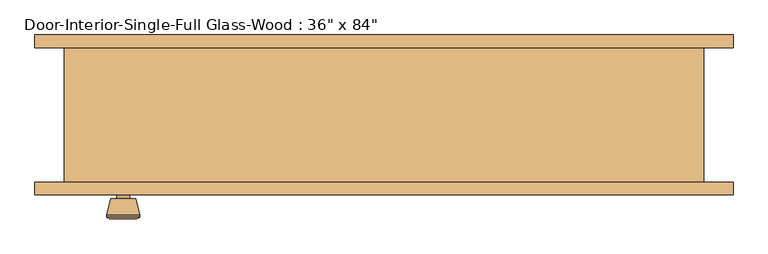
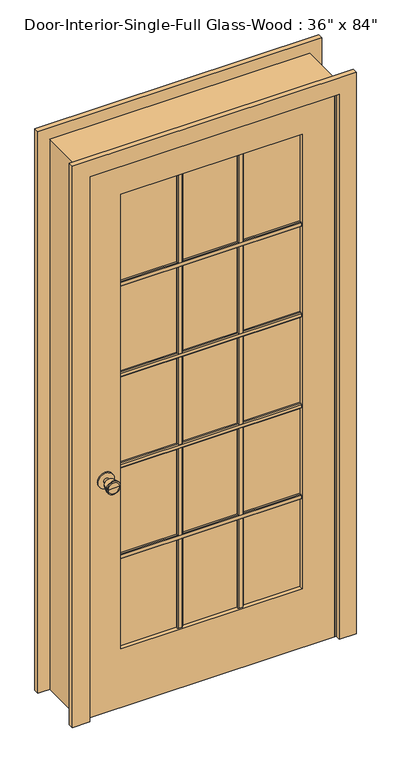
"""IFC4 building model written with IfcOpenShell, lengths in millimetres: door geometry."""

from ifc_helpers import new_model, si_unit, point, frame, frame_2d, origin, place, context, project, spatial, polyline, circle_curve, trimmed, segment, composite_curve, outline, extrude, faceted_brep, source, transform, mapped, element, save
from ifc_brep_helpers import plane_surface, cylinder_surface, revolved_surface, advanced_brep


def door_6e1855c2(model_context):
    return source(origin(), model_context, "Body", "SolidModel", [
        extrude(outline(polyline([(-84.455, 1667.51), (-84.455, 1648.46), (-90.805, 1648.46), (-93.98, 1651.635), (-93.98, 1664.335), (-90.805, 1667.51), (-84.455, 1667.51)])), frame((-336.55, 0.0, 0.0), z_axis=(1.0, 0.0, 0.0), x_axis=(0.0, 1.0, 0.0)), (0.0, 0.0, 1.0), 673.1),
        extrude(outline(polyline([(-84.455, 1310.9575), (-84.455, 1291.9075), (-90.805, 1291.9075), (-93.98, 1295.0825), (-93.98, 1307.7825), (-90.805, 1310.9575), (-84.455, 1310.9575)])), frame((-336.55, 0.0, 0.0), z_axis=(1.0, 0.0, 0.0), x_axis=(0.0, 1.0, 0.0)), (0.0, 0.0, 1.0), 673.1),
        extrude(outline(polyline([(-84.455, 954.405), (-84.455, 935.355), (-90.805, 935.355), (-93.98, 938.53), (-93.98, 951.23), (-90.805, 954.405), (-84.455, 954.405)])), frame((-336.55, 0.0, 0.0), z_axis=(1.0, 0.0, 0.0), x_axis=(0.0, 1.0, 0.0)), (0.0, 0.0, 1.0), 673.1),
        extrude(outline(polyline([(-84.455, 597.8525), (-84.455, 578.8025), (-90.805, 578.8025), (-93.98, 581.9775), (-93.98, 594.6775), (-90.805, 597.8525), (-84.455, 597.8525)])), frame((-336.55, 0.0, 0.0), z_axis=(1.0, 0.0, 0.0), x_axis=(0.0, 1.0, 0.0)), (0.0, 0.0, 1.0), 673.1),
        extrude(outline(polyline([(102.6583333, -84.455), (121.7083333, -84.455), (121.7083333, -90.805), (118.5333333, -93.98), (105.8333333, -93.98), (102.6583333, -90.805), (102.6583333, -84.455)])), frame((0.0, 0.0, 231.775), z_axis=(0.0, 0.0, 1.0), x_axis=(1.0, 0.0, 0.0)), (0.0, 0.0, 1.0), 1782.7625),
        extrude(outline(polyline([(-121.7083333, -84.455), (-102.6583333, -84.455), (-102.6583333, -90.805), (-105.8333333, -93.98), (-118.5333333, -93.98), (-121.7083333, -90.805), (-121.7083333, -84.455)])), frame((0.0, 0.0, 231.775), z_axis=(0.0, 0.0, 1.0), x_axis=(1.0, 0.0, 0.0)), (0.0, 0.0, 1.0), 1782.7625),
        extrude(outline(polyline([(-77.47, 1667.51), (-71.12, 1667.51), (-67.945, 1664.335), (-67.945, 1651.635), (-71.12, 1648.46), (-77.47, 1648.46), (-77.47, 1667.51)])), frame((-336.55, 0.0, 0.0), z_axis=(1.0, 0.0, 0.0), x_axis=(0.0, 1.0, 0.0)), (0.0, 0.0, 1.0), 673.1),
        extrude(outline(polyline([(-77.47, 1310.9575), (-71.12, 1310.9575), (-67.945, 1307.7825), (-67.945, 1295.0825), (-71.12, 1291.9075), (-77.47, 1291.9075), (-77.47, 1310.9575)])), frame((-336.55, 0.0, 0.0), z_axis=(1.0, 0.0, 0.0), x_axis=(0.0, 1.0, 0.0)), (0.0, 0.0, 1.0), 673.1),
        extrude(outline(polyline([(-77.47, 954.405), (-71.12, 954.405), (-67.945, 951.23), (-67.945, 938.53), (-71.12, 935.355), (-77.47, 935.355), (-77.47, 954.405)])), frame((-336.55, 0.0, 0.0), z_axis=(1.0, 0.0, 0.0), x_axis=(0.0, 1.0, 0.0)), (0.0, 0.0, 1.0), 673.1),
        extrude(outline(polyline([(-77.47, 597.8525), (-71.12, 597.8525), (-67.945, 594.6775), (-67.945, 581.9775), (-71.12, 578.8025), (-77.47, 578.8025), (-77.47, 597.8525)])), frame((-336.55, 0.0, 0.0), z_axis=(1.0, 0.0, 0.0), x_axis=(0.0, 1.0, 0.0)), (0.0, 0.0, 1.0), 673.1),
        extrude(outline(polyline([(102.6583333, -77.47), (102.6583333, -71.12), (105.8333333, -67.945), (118.5333333, -67.945), (121.7083333, -71.12), (121.7083333, -77.47), (102.6583333, -77.47)])), frame((0.0, 0.0, 231.775), z_axis=(0.0, 0.0, 1.0), x_axis=(1.0, 0.0, 0.0)), (0.0, 0.0, 1.0), 1782.7625),
        extrude(outline(polyline([(-121.7083333, -77.47), (-121.7083333, -71.12), (-118.5333333, -67.945), (-105.8333333, -67.945), (-102.6583333, -71.12), (-102.6583333, -77.47), (-121.7083333, -77.47)])), frame((0.0, 0.0, 231.775), z_axis=(0.0, 0.0, 1.0), x_axis=(1.0, 0.0, 0.0)), (0.0, 0.0, 1.0), 1782.7625),
        advanced_brep(
        [(-393.7, -57.5, 914.4), (-403.7, -57.5, 914.4), (-383.7, -57.5, 914.4), (-373.2241324, -8.5, 914.4), (-414.1758676, -8.5, 914.4), (-393.7, -8.5, 914.4), (-368.7, -10.3278681, 914.4), (-418.7, -10.3278681, 914.4), (-368.7, -13.7915463, 914.4), (-418.7, -13.7915463, 914.4), (-375.063764, -38.5, 914.4), (-412.336236, -38.5, 914.4), (-383.7, -38.5, 914.4), (-403.7, -38.5, 914.4)],
        [
            (0, 1),
            (1, 2, circle_curve(frame((-393.7, -57.5, 914.4), z_axis=(0.0, -1.0, 0.0), x_axis=(-1.0, 0.0, 0.0)), 10.0)),
            (2, 0),
            (2, 1, circle_curve(frame((-393.7, -57.5, 914.4), z_axis=(0.0, -1.0, 0.0), x_axis=(-1.0, 0.0, 0.0)), 10.0)),
            (3, 4, circle_curve(frame((-393.7, -8.5, 914.4), z_axis=(0.0, 1.0, 0.0), x_axis=(-1.0, 0.0, 0.0)), 20.4758676)),
            (4, 5),
            (5, 3),
            (4, 3, circle_curve(frame((-393.7, -8.5, 914.4), z_axis=(0.0, 1.0, 0.0), x_axis=(-1.0, 0.0, 0.0)), 20.4758676)),
            (6, 7, circle_curve(frame((-393.7, -10.3278681, 914.4), z_axis=(0.0, 1.0, 0.0), x_axis=(-1.0, 0.0, 0.0)), 25.0)),
            (7, 4),
            (3, 6),
            (7, 6, circle_curve(frame((-393.7, -10.3278681, 914.4), z_axis=(0.0, 1.0, 0.0), x_axis=(-1.0, 0.0, 0.0)), 25.0)),
            (8, 9, circle_curve(frame((-393.7, -13.7915463, 914.4), z_axis=(0.0, 1.0, 0.0), x_axis=(-1.0, 0.0, 0.0)), 25.0)),
            (9, 7),
            (6, 8),
            (9, 8, circle_curve(frame((-393.7, -13.7915463, 914.4), z_axis=(0.0, 1.0, 0.0), x_axis=(-1.0, 0.0, 0.0)), 25.0)),
            (10, 11, circle_curve(frame((-393.7, -38.5, 914.4), z_axis=(0.0, 1.0, 0.0), x_axis=(-1.0, 0.0, 0.0)), 18.636236)),
            (11, 9),
            (8, 10),
            (11, 10, circle_curve(frame((-393.7, -38.5, 914.4), z_axis=(0.0, 1.0, 0.0), x_axis=(-1.0, 0.0, 0.0)), 18.636236)),
            (12, 13, circle_curve(frame((-393.7, -38.5, 914.4), z_axis=(0.0, 1.0, 0.0), x_axis=(-1.0, 0.0, 0.0)), 10.0)),
            (13, 11),
            (10, 12),
            (13, 12, circle_curve(frame((-393.7, -38.5, 914.4), z_axis=(0.0, 1.0, 0.0), x_axis=(-1.0, 0.0, 0.0)), 10.0)),
            (1, 13),
            (12, 2),
        ],
        [
            plane_surface(frame((-393.7, -57.5, 914.4), z_axis=(0.0, -1.0, 0.0), x_axis=(-1.0, 0.0, 0.0))),
            plane_surface(frame((-393.7, -8.5, 914.4), z_axis=(0.0, 1.0, 0.0), x_axis=(-1.0, 0.0, 0.0))),
            revolved_surface(polyline([(-414.1758676, -8.5, 914.4), (-418.7, -10.3278681, 914.4)]), (-393.7, -57.5, 914.4), (0.0, -1.0, 0.0)),
            cylinder_surface(frame((-393.7, -57.5, 914.4), z_axis=(0.0, -1.0, 0.0), x_axis=(-1.0, 0.0, 0.0)), 25.0),
            revolved_surface(polyline([(-418.7, -13.7915463, 914.4), (-412.336236, -38.5, 914.4)]), (-393.7, -57.5, 914.4), (0.0, -1.0, 0.0)),
            plane_surface(frame((-393.7, -38.5, 914.4), z_axis=(0.0, -1.0, 0.0), x_axis=(-1.0, 0.0, 0.0))),
            cylinder_surface(frame((-393.7, -57.5, 914.4), z_axis=(0.0, -1.0, 0.0), x_axis=(-1.0, 0.0, 0.0)), 10.0),
        ],
        [
            (0, [[1, 2, 3]]),
            (0, [[-3, 4, -1]]),
            (1, [[5, 6, 7]]),
            (1, [[8, -7, -6]]),
            (2, [[9, 10, -5, 11]]),
            (2, [[12, -11, -8, -10]]),
            (3, [[13, 14, -9, 15]]),
            (3, [[16, -15, -12, -14]]),
            (4, [[17, 18, -13, 19]]),
            (4, [[20, -19, -16, -18]]),
            (5, [[21, 22, -17, 23]]),
            (5, [[24, -23, -20, -22]]),
            (6, [[-2, 25, -21, 26]]),
            (6, [[-4, -26, -24, -25]]),
        ],
    ),
        extrude(outline(composite_curve([segment(trimmed(circle_curve(frame_2d((914.4, -393.7)), 30.0), [point((914.4, -423.7))], [point((914.4, -363.7))], False, "CARTESIAN"), True, "CONTINUOUS"), segment(trimmed(circle_curve(frame_2d((914.4, -393.7)), 30.0), [point((914.4, -363.7))], [point((914.4, -423.7))], False, "CARTESIAN"), True, "CONTINUOUS")], self_intersect=False)), frame((0.0, -63.5, 0.0), z_axis=(0.0, 1.0, 0.0), x_axis=(0.0, 0.0, 1.0)), (0.0, 0.0, 1.0), 6.0),
        advanced_brep(
        [(-393.7, -104.425, 914.4), (-383.7, -104.425, 914.4), (-403.7, -104.425, 914.4), (-373.2241324, -153.425, 914.4), (-393.7, -153.425, 914.4), (-414.1758676, -153.425, 914.4), (-368.7, -151.5971319, 914.4), (-418.7, -151.5971319, 914.4), (-368.7, -148.1334537, 914.4), (-418.7, -148.1334537, 914.4), (-375.063764, -123.425, 914.4), (-412.336236, -123.425, 914.4), (-383.7, -123.425, 914.4), (-403.7, -123.425, 914.4)],
        [
            (0, 1),
            (1, 2, circle_curve(frame((-393.7, -104.425, 914.4), z_axis=(0.0, 1.0, 0.0), x_axis=(-1.0, 0.0, 0.0)), 10.0)),
            (2, 0),
            (2, 1, circle_curve(frame((-393.7, -104.425, 914.4), z_axis=(0.0, 1.0, 0.0), x_axis=(-1.0, 0.0, 0.0)), 10.0)),
            (3, 4),
            (4, 5),
            (5, 3, circle_curve(frame((-393.7, -153.425, 914.4), z_axis=(0.0, -1.0, 0.0), x_axis=(-1.0, 0.0, 0.0)), 20.4758676)),
            (3, 5, circle_curve(frame((-393.7, -153.425, 914.4), z_axis=(0.0, -1.0, 0.0), x_axis=(-1.0, 0.0, 0.0)), 20.4758676)),
            (6, 3),
            (5, 7),
            (7, 6, circle_curve(frame((-393.7, -151.5971319, 914.4), z_axis=(0.0, -1.0, 0.0), x_axis=(-1.0, 0.0, 0.0)), 25.0)),
            (6, 7, circle_curve(frame((-393.7, -151.5971319, 914.4), z_axis=(0.0, -1.0, 0.0), x_axis=(-1.0, 0.0, 0.0)), 25.0)),
            (8, 6),
            (7, 9),
            (9, 8, circle_curve(frame((-393.7, -148.1334537, 914.4), z_axis=(0.0, -1.0, 0.0), x_axis=(-1.0, 0.0, 0.0)), 25.0)),
            (8, 9, circle_curve(frame((-393.7, -148.1334537, 914.4), z_axis=(0.0, -1.0, 0.0), x_axis=(-1.0, 0.0, 0.0)), 25.0)),
            (10, 8),
            (9, 11),
            (11, 10, circle_curve(frame((-393.7, -123.425, 914.4), z_axis=(0.0, -1.0, 0.0), x_axis=(-1.0, 0.0, 0.0)), 18.636236)),
            (10, 11, circle_curve(frame((-393.7, -123.425, 914.4), z_axis=(0.0, -1.0, 0.0), x_axis=(-1.0, 0.0, 0.0)), 18.636236)),
            (12, 10),
            (11, 13),
            (13, 12, circle_curve(frame((-393.7, -123.425, 914.4), z_axis=(0.0, -1.0, 0.0), x_axis=(-1.0, 0.0, 0.0)), 10.0)),
            (12, 13, circle_curve(frame((-393.7, -123.425, 914.4), z_axis=(0.0, -1.0, 0.0), x_axis=(-1.0, 0.0, 0.0)), 10.0)),
            (1, 12),
            (13, 2),
        ],
        [
            plane_surface(frame((-393.7, -104.425, 914.4), z_axis=(0.0, 1.0, 0.0), x_axis=(-1.0, 0.0, 0.0))),
            plane_surface(frame((-393.7, -153.425, 914.4), z_axis=(0.0, -1.0, 0.0), x_axis=(-1.0, 0.0, 0.0))),
            revolved_surface(polyline([(-414.1758676, -153.425, 914.4), (-418.7, -151.5971319, 914.4)]), (-393.7, -104.425, 914.4), (0.0, 1.0, 0.0)),
            cylinder_surface(frame((-393.7, -104.425, 914.4), z_axis=(0.0, 1.0, 0.0), x_axis=(-1.0, 0.0, 0.0)), 25.0),
            revolved_surface(polyline([(-418.7, -148.1334537, 914.4), (-412.336236, -123.425, 914.4)]), (-393.7, -104.425, 914.4), (0.0, 1.0, 0.0)),
            plane_surface(frame((-393.7, -123.425, 914.4), z_axis=(0.0, 1.0, 0.0), x_axis=(-1.0, 0.0, 0.0))),
            cylinder_surface(frame((-393.7, -104.425, 914.4), z_axis=(0.0, 1.0, 0.0), x_axis=(-1.0, 0.0, 0.0)), 10.0),
        ],
        [
            (0, [[1, 2, 3]]),
            (0, [[-3, 4, -1]]),
            (1, [[5, 6, 7]]),
            (1, [[-6, -5, 8]]),
            (2, [[9, -7, 10, 11]]),
            (2, [[-10, -8, -9, 12]]),
            (3, [[13, -11, 14, 15]]),
            (3, [[-14, -12, -13, 16]]),
            (4, [[17, -15, 18, 19]]),
            (4, [[-18, -16, -17, 20]]),
            (5, [[21, -19, 22, 23]]),
            (5, [[-22, -20, -21, 24]]),
            (6, [[25, -23, 26, -2]]),
            (6, [[-26, -24, -25, -4]]),
        ],
    ),
        extrude(outline(composite_curve([segment(trimmed(circle_curve(frame_2d((914.4, -393.7)), 30.0), [point((914.4, -423.7))], [point((914.4, -363.7))], False, "CARTESIAN"), True, "CONTINUOUS"), segment(trimmed(circle_curve(frame_2d((914.4, -393.7)), 30.0), [point((914.4, -363.7))], [point((914.4, -423.7))], False, "CARTESIAN"), True, "CONTINUOUS")], self_intersect=False)), frame((0.0, -104.425, 0.0), z_axis=(0.0, 1.0, 0.0), x_axis=(0.0, 0.0, 1.0)), (0.0, 0.0, 1.0), 6.0),
        extrude(outline(polyline([(2133.6, -457.2), (0.0, -457.2), (0.0, 457.2), (2133.6, 457.2), (2133.6, -457.2)]), holes=[polyline([(2014.5375, -336.55), (2014.5375, 336.55), (231.775, 336.55), (231.775, -336.55), (2014.5375, -336.55)])]), frame((0.0, -98.425, 0.0), z_axis=(0.0, 1.0, 0.0), x_axis=(0.0, 0.0, 1.0)), (0.0, 0.0, 1.0), 34.925),
        faceted_brep([(482.6, -98.425, 0.0), (457.2, -98.425, 0.0), (457.2, -63.5, 0.0), (444.5, -63.5, 0.0), (444.5, -28.575, 0.0), (457.2, -28.575, 0.0), (457.2, 104.775, 0.0), (482.6, 104.775, 0.0), (482.6, 104.775, 2159.0), (482.6, -98.425, 2159.0), (457.2, 104.775, 2133.6), (-457.2, 104.775, 2133.6), (-457.2, 104.775, 0.0), (-482.6, 104.775, 0.0), (-482.6, 104.775, 2159.0), (457.2, -28.575, 2133.6), (444.5, -28.575, 2120.9), (-444.5, -28.575, 2120.9), (-444.5, -28.575, 0.0), (-457.2, -28.575, 0.0), (-457.2, -28.575, 2133.6), (444.5, -63.5, 2120.9), (457.2, -63.5, 2133.6), (-457.2, -63.5, 2133.6), (-457.2, -63.5, 0.0), (-444.5, -63.5, 0.0), (-444.5, -63.5, 2120.9), (457.2, -98.425, 2133.6), (-482.6, -98.425, 2159.0), (-482.6, -98.425, 0.0), (-457.2, -98.425, 0.0), (-457.2, -98.425, 2133.6)], [[[0, 1, 2, 3, 4, 5, 6, 7]], [[7, 8, 9, 0]], [[6, 10, 11, 12, 13, 14, 8, 7]], [[5, 15, 10, 6]], [[4, 16, 17, 18, 19, 20, 15, 5]], [[3, 21, 16, 4]], [[2, 22, 23, 24, 25, 26, 21, 3]], [[1, 27, 22, 2]], [[0, 9, 28, 29, 30, 31, 27, 1]], [[8, 14, 28, 9]], [[15, 20, 11, 10]], [[21, 26, 17, 16]], [[27, 31, 23, 22]], [[29, 13, 12, 19, 18, 25, 24, 30]], [[14, 13, 29, 28]], [[20, 19, 12, 11]], [[26, 25, 18, 17]], [[31, 30, 24, 23]]]),
        extrude(outline(polyline([(336.55, -77.47), (336.55, -84.455), (-336.55, -84.455), (-336.55, -77.47), (336.55, -77.47)])), frame((0.0, 0.0, 231.775), z_axis=(0.0, 0.0, 1.0), x_axis=(1.0, 0.0, 0.0)), (0.0, 0.0, 1.0), 1782.7625),
        extrude(outline(polyline([(0.0, 527.05), (2203.45, 527.05), (2203.45, -527.05), (0.0, -527.05), (0.0, -463.55), (2139.95, -463.55), (2139.95, 463.55), (0.0, 463.55), (0.0, 527.05)])), frame((0.0, 104.775, 0.0), z_axis=(0.0, 1.0, 0.0), x_axis=(0.0, 0.0, 1.0)), (0.0, 0.0, 1.0), 19.05),
        extrude(outline(polyline([(0.0, 527.05), (2203.45, 527.05), (2203.45, -527.05), (0.0, -527.05), (0.0, -463.55), (2139.95, -463.55), (2139.95, 463.55), (0.0, 463.55), (0.0, 527.05)])), frame((0.0, -117.475, 0.0), z_axis=(0.0, 1.0, 0.0), x_axis=(0.0, 0.0, 1.0)), (0.0, 0.0, 1.0), 19.05),
    ])


if __name__ == "__main__":
    model = new_model("IFC4")
    model_context = context("Model", 3, world=origin())
    ifc_project = project(units=[si_unit("LENGTHUNIT", "METRE", prefix="MILLI")], contexts=[model_context])
    site = spatial("IfcSite", under=ifc_project)
    building = spatial("IfcBuilding", under=site)
    placement = place(None, origin())
    door_shape = door_6e1855c2(model_context)
    element("IfcDoor", 1, ObjectType="Door-Interior-Single-Full Glass-Wood : 36\" x 84\"", at=placement, inside=building, context=model_context, shape_type="MappedRepresentation", body=[
        mapped(door_shape, transform((0.0, 0.0, 0.0), x_axis=(1.0, 0.0, 0.0), y_axis=(0.0, 1.0, 0.0), z_axis=(0.0, 0.0, 1.0))),
    ])
    save(model, "model.ifc")

# Revit data of these elements
# Type "Door-Interior-Single-Full Glass-Wood : 36\" x 84\""
#   Type Mark = "11"
#   Assembly Code = "C1020300"
#   Analytic Construction = "Wood frame with single clear glass"
#   Top Rail = 0' - 4 11/16"
#   Thickness = 0' - 1 3/8"
#   Thermal Resistance (R) = 1.0102 (h·ft²·°F)/BTU
#   Swing Angle [instance default] = 90.00°
#   Stiles = 0' - 4 3/4"
#   Rough Width = 3' - 2"
#   Rough Height = 7' - 1"
#   Height = 7' - 0"
#   Width = 3' - 0"
#   Heat Transfer Coefficient (U) = 0.9900 BTU/(h·ft²·°F)
#   Bottom Rail = 0' - 9 1/8"
#   Show Grill [instance default] = yes
#   Trim Material = Cherry
#   Panel Material = Cherry
#   Frame Material = Cherry
#   Door Handle Material = Aluminum
#   Visual Light Transmittance = 0
#   Solar Heat Gain Coefficient = 0
#   Wall Closure = (empty or 0)
#   Function = (empty or 0)
# Element 1 (IfcDoor, "Door-Interior-Single-Full Glass-Wood : 36\" x 84\"")
#   Materials on its faces: "Cherry", "Aluminum", "Glass"
# Materials
#   "Cherry": class "Wood", colour RGB 226 177 128, transparency 0, Description = "Prunus Serotina", Cost = 0
#   "Aluminum": class "Metal", colour RGB 247 247 247, transparency 0, Description = "Aluminum 6061", Cost = 0
#   "Glass": class "Glass", colour RGB 0 128 192, transparency 0.75, Description = "Soda Lime Glass", Cost = 0
